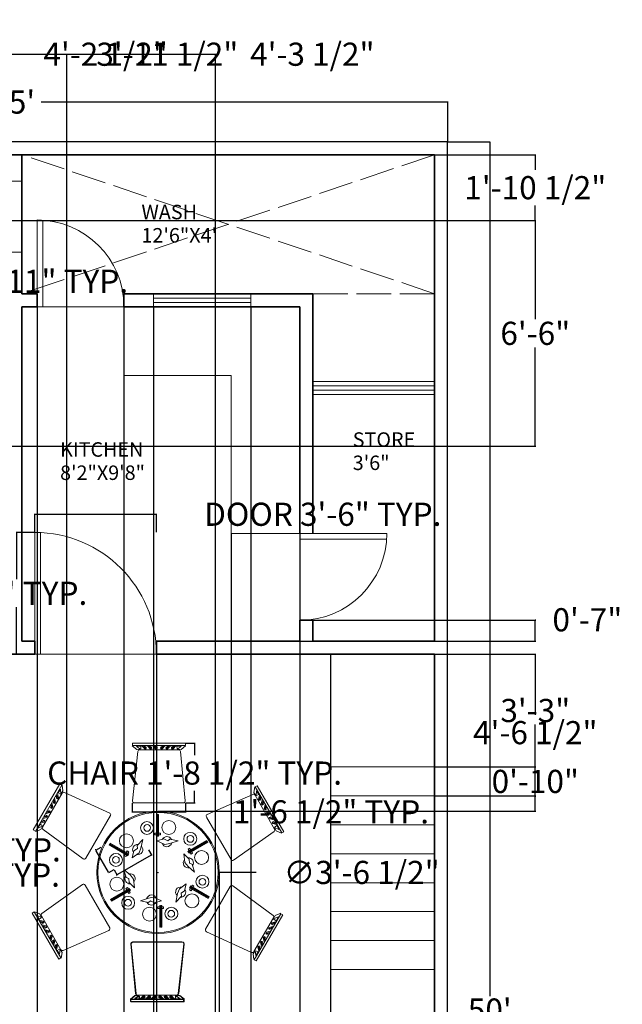
# Model space of a CAD drawing. Units: inches. Extents: x -26 to 385, y 12 to 697.
# Tile 13 of 13: x 177 to 385, y 356 to 697. Entities that reach past the tile are written whole.
import ezdxf

# ---------------------------------------------------------------- set-up
doc = ezdxf.new("R2010")
doc.units = ezdxf.units.IN
doc.header["$MEASUREMENT"] = 0
doc.linetypes.add('ACAD_ISO02W100', pattern=[15, 12, -3])
for name, color, linetype, lineweight in [('A-ANNO-DIMS', 4, 'Continuous', 18), ('A-AREA-IDEN', 4, 'Continuous', 18), ('A-DOOR', 30, 'Continuous', 20), ('A-FLOR-CASE', 7, 'Continuous', 18), ('A-FLOR-OVHD', 3, 'ACAD_ISO02W100', 13), ('A-FLOR-STRS', 215, 'Continuous', 18), ('A-GLAZ', 5, 'Continuous', 18), ('A-WALL', 40, 'Continuous', 35), ('C-PROP', 40, 'Continuous', 25), ('Furniture', 210, 'Continuous', 15)]:
    doc.layers.add(name, color=color, linetype=linetype, lineweight=lineweight)
doc.styles.get("Standard").update_dxf_attribs({"font": 'italic8.shx'})
doc.dimstyles.get("Standard").update_dxf_attribs({"dimtxt": 8, "dimasz": 0.18, "dimexe": 0.18, "dimexo": 0.0625, "dimgap": 0.09, "dimtad": 0, "dimtih": 1, "dimtoh": 1, "dimdec": 4, "dimzin": 0, "dimdsep": 46, "dimlunit": 3, "dimtxsty": 'Standard', "dimcen": 0.09, "dimclrd": 2, "dimclre": 3, "dimclrt": 6, "dimadec": 0, "dimazin": 0, "dimtfac": 1, "dimtdec": 4, "dimtofl": 0, "dimtmove": 0, "dimatfit": 3, "dimfxl": 1, "dimtolj": 1, "dimtzin": 0, "dimarcsym": 0})

# ---------------------------------------------------------------- blocks, each defined once
blk = doc.blocks.new('*D1')
at = {"layer": 'A-ANNO-DIMS', "color": 0, "lineweight": -2, "transparency": 16777216}
for p, q in [((25.13, 654.44), (25.13, 668.29)), ((25.31, 668.11), (165.52, 668.11)), ((324.95, 668.11), (184.74, 668.11)), ((325.13, 654.44), (325.13, 668.29))]:
    blk.add_line(p, q, dxfattribs=at)
at = {"layer": 'A-ANNO-DIMS', "color": 0, "transparency": 16777216}
for points in [[(25.31, 668.14), (25.31, 668.08), (25.13, 668.11)], [(324.95, 668.14), (324.95, 668.08), (325.13, 668.11)]]:
    blk.add_solid(points, dxfattribs=at)
at = {"layer": 'Defpoints', "color": 0, "transparency": 16777216}
for p in [(325.13, 668.11), (25.13, 654.38), (325.13, 654.38)]:
    blk.add_point(p, dxfattribs=at)
at = {"layer": 'A-ANNO-DIMS', "color": 0, "transparency": 16777216, "insert": (175.13, 668.11), "char_height": 8, "attachment_point": 5}
blk.add_mtext("\\A1;25'", dxfattribs=at)
blk = doc.blocks.new('*D2')
at = {"layer": 'A-ANNO-DIMS', "color": 0, "lineweight": -2, "transparency": 16777216}
for p, q in [((325.19, 654.38), (339.84, 654.38)), ((339.66, 654.2), (339.66, 359.23)), ((339.66, 54.56), (339.66, 349.53)), ((325.19, 54.38), (339.84, 54.38))]:
    blk.add_line(p, q, dxfattribs=at)
at = {"layer": 'A-ANNO-DIMS', "color": 0, "transparency": 16777216}
for points in [[(339.63, 654.2), (339.69, 654.2), (339.66, 654.38)], [(339.63, 54.56), (339.69, 54.56), (339.66, 54.38)]]:
    blk.add_solid(points, dxfattribs=at)
at = {"layer": 'Defpoints', "color": 0, "transparency": 16777216}
for p in [(325.13, 654.38), (325.13, 54.38), (339.66, 54.38)]:
    blk.add_point(p, dxfattribs=at)
at = {"layer": 'A-ANNO-DIMS', "color": 0, "transparency": 16777216, "insert": (339.66, 354.38), "char_height": 8, "attachment_point": 5}
blk.add_mtext("\\A1;50'", dxfattribs=at)
blk = doc.blocks.new('DOOR-SWING-30IN')
for p, q in [((0, -30), (0, 0)), ((0, 0), (30, 0)), ((0, -2), (30, -2))]:
    blk.add_line(p, q)
blk.add_arc((0, 0), 30, 270, 0)
blk = doc.blocks.new('DOOR-SWING-42IN')
for p, q in [((0, 0), (0, 42)), ((2, 0), (2, 42)), ((42, 0), (0, 0))]:
    blk.add_line(p, q)
blk.add_arc((0, 0), 42, 0, 90)
blk = doc.blocks.new('CHAIR-DINING')
for p, q in [((-17.53, 10.49), (-15.96, 9.24)), ((-17.41, 11.37), (-17.41, 10.56)), ((0.95, 11.37), (-17.41, 11.37)), ((-17.41, 10.56), (0.95, 10.56)), ((-16.02, 10.31), (-14.51, 10.37)), ((-14.64, 9.3), (-16.02, 10.31)), ((-14.51, 10.37), (-14.58, 9.49)), ((-14.14, 10.43), (-13.19, 9.49)), ((-13.63, 10.37), (-13.26, 10.37)), ((-12.69, 9.49), (-13.63, 10.37)), ((-13.26, 10.37), (-12.82, 9.99)), ((-12.25, 10.43), (-11.31, 9.49)), ((-11.75, 10.37), (-11.37, 10.37)), ((-10.81, 9.49), (-11.75, 10.37)), ((-11.37, 10.37), (-10.93, 9.99)), ((-10.37, 10.43), (-9.42, 9.49)), ((-9.86, 10.37), (-9.49, 10.37)), ((-8.92, 9.49), (-9.86, 10.37)), ((-9.49, 10.37), (-9.05, 9.99)), ((-7.66, 9.49), (-6.72, 10.37)), ((-7.1, 10.37), (-7.54, 9.99)), ((-6.22, 10.43), (-7.16, 9.49)), ((-6.72, 10.37), (-7.1, 10.37)), ((-5.78, 9.49), (-4.83, 10.37)), ((-5.21, 10.37), (-5.65, 9.99)), ((-4.33, 10.43), (-5.27, 9.49)), ((-4.83, 10.37), (-5.21, 10.37)), ((-3.89, 9.49), (-2.95, 10.37)), ((-3.33, 10.37), (-3.77, 9.99)), ((-2.45, 10.43), (-3.39, 9.49)), ((-2.95, 10.37), (-3.33, 10.37)), ((-2.07, 10.37), (-2.01, 9.49)), ((-0.56, 10.31), (-2.07, 10.37)), ((-1.94, 9.3), (-0.56, 10.31)), ((0.95, 10.49), (-0.62, 9.24)), ((0.95, 10.56), (0.95, 11.37)), ((-17.45, -8.54), (-15.58, 8.55)), ((-15.96, 9.24), (-14.64, 9.3)), ((-14.96, 9.11), (-1.45, 9.11)), ((-13.19, 9.49), (-12.69, 9.49)), ((-12.82, 9.99), (-12.69, 10.12)), ((-12.69, 10.12), (-12.63, 9.55)), ((-11.31, 9.49), (-10.81, 9.49)), ((-10.93, 9.99), (-10.81, 10.12)), ((-10.81, 10.12), (-10.74, 9.55)), ((-9.42, 9.49), (-8.92, 9.49)), ((-9.05, 9.99), (-8.92, 10.12)), ((-8.92, 10.12), (-8.86, 9.55)), ((-7.66, 10.12), (-7.73, 9.55)), ((-7.54, 9.99), (-7.66, 10.12)), ((-7.16, 9.49), (-7.66, 9.49)), ((-5.78, 10.12), (-5.84, 9.55)), ((-5.65, 9.99), (-5.78, 10.12)), ((-5.27, 9.49), (-5.78, 9.49)), ((-3.89, 10.12), (-3.95, 9.55)), ((-3.77, 9.99), (-3.89, 10.12)), ((-3.39, 9.49), (-3.89, 9.49)), ((-0.62, 9.24), (-1.94, 9.3)), ((-0.82, 8.54), (0.82, -8.54)), ((0.19, -9.23), (-16.83, -9.23))]:
    blk.add_line(p, q)
for centre, start, end in [((-14.96, 8.48), 90, 173.7428), ((-1.45, 8.48), 5.4801, 90), ((-16.83, -8.6), 173.7428, 270), ((0.19, -8.6), 270, 5.4801)]:
    blk.add_arc(centre, 0.629, start, end)
blk = doc.blocks.new('DINING-PLACE-SETTING')
for p, q in [((5.72, -0.56, 3.57), (-0.79, -4.32, 3.57)), ((-0.18, -3.27, 3.57), (-0.71, -3.57, 3.57)), ((-0.67, -4.53, 3.57), (5.84, -0.77, 3.57)), ((5.95, -0.95, 3.57), (-0.56, -4.71, 3.57)), ((-0.45, -4.91, 3.57), (6.06, -1.15, 3.57)), ((0.13, -3.79, 3.57), (-0.18, -3.27, 3.57)), ((5.84, -0.77, 3.57), (5.72, -0.56, 3.57)), ((6.06, -1.15, 3.57), (5.95, -0.95, 3.57)), ((-0.34, -6.97, 3.57), (-2.16, -5.22, 3.57)), ((-2.16, -5.22, 3.57), (-1.81, -8.16, 3.57)), ((-0.79, -4.32, 3.57), (-0.67, -4.53, 3.57)), ((-0.71, -3.57, 3.57), (-0.4, -4.1, 3.57)), ((-0.56, -4.71, 3.57), (-0.45, -4.91, 3.57)), ((-0.28, -4.3, 3.57), (-0.18, -4.49, 3.57)), ((-0.06, -4.69, 3.57), (0.27, -5.26, 3.57)), ((0.35, -4.18, 3.57), (0.24, -4, 3.57)), ((0.27, -5.26, 3.57), (0.8, -4.96, 3.57)), ((0.8, -4.96, 3.57), (0.47, -4.39, 3.57)), ((-1.81, -8.16, 3.57), (-0.75, -9.53, 3.57)), ((-0.75, -9.53, 3.57), (1.48, -11.52, 3.57)), ((-0.22, -8.41, 3.57), (-0.34, -6.97, 3.57)), ((0.67, -8.78, 3.57), (-0.22, -8.41, 3.57)), ((1.48, -11.52, 3.57), (0.67, -8.78, 3.57))]:
    blk.add_line(p, q)
for centre, radius in [((0, 0, 3.57), 2.24), ((0.05, -0.03, 3.57), 1.16), ((3.93, -6.44, 3.57), 2.41)]:
    blk.add_circle(centre, radius)
for start, end in [(326.6641, 94.1442), (137.0611, 284.0662)]:
    blk.add_arc((-0.65, -8.3, 3.57), 1.75, start, end)
blk = doc.blocks.new('*D13')
at = {"layer": 'A-ANNO-DIMS', "color": 3, "lineweight": -2, "transparency": 16777216}
for p, q in [((234.73, 446.56), (237.94, 446.56)), ((234.73, 425.95), (237.94, 425.95))]:
    blk.add_line(p, q, dxfattribs=at)
at = {"layer": 'A-ANNO-DIMS', "color": 2, "lineweight": -2, "transparency": 16777216}
for p, q in [((237.76, 446.38), (237.76, 442.44)), ((237.76, 426.13), (237.76, 430.07))]:
    blk.add_line(p, q, dxfattribs=at)
at = {"layer": 'A-ANNO-DIMS', "color": 2, "transparency": 16777216}
for points in [[(237.73, 446.38), (237.79, 446.38), (237.76, 446.56)], [(237.73, 426.13), (237.79, 426.13), (237.76, 425.95)]]:
    blk.add_solid(points, dxfattribs=at)
at = {"layer": 'Defpoints', "color": 0, "transparency": 16777216}
for p in [(234.67, 446.56), (237.76, 446.56), (234.67, 425.95)]:
    blk.add_point(p, dxfattribs=at)
at = {"layer": 'A-ANNO-DIMS', "color": 6, "transparency": 16777216, "insert": (237.76, 436.26), "char_height": 8, "attachment_point": 5}
blk.add_mtext('\\A1;CHAIR 1\'-8 1/2" TYP.', dxfattribs=at)
blk = doc.blocks.new('*D14')
at = {"layer": 'A-ANNO-DIMS', "color": 3, "lineweight": -2, "transparency": 16777216}
for p, q in [((216.19, 425.89), (216.19, 422.68)), ((234.67, 425.89), (234.67, 422.68))]:
    blk.add_line(p, q, dxfattribs=at)
at = {"layer": 'A-ANNO-DIMS', "color": 2, "lineweight": -2, "transparency": 16777216}
for p, q in [((216.37, 422.86), (234.49, 422.86)), ((234.67, 422.86), (234.85, 422.86))]:
    blk.add_line(p, q, dxfattribs=at)
at = {"layer": 'A-ANNO-DIMS', "color": 2, "transparency": 16777216}
for points in [[(216.37, 422.89), (216.37, 422.83), (216.19, 422.86)], [(234.49, 422.89), (234.49, 422.83), (234.67, 422.86)]]:
    blk.add_solid(points, dxfattribs=at)
at = {"layer": 'Defpoints', "color": 0, "transparency": 16777216}
for p in [(216.19, 425.95), (234.67, 425.95), (234.67, 422.86)]:
    blk.add_point(p, dxfattribs=at)
at = {"layer": 'A-ANNO-DIMS', "color": 6, "transparency": 16777216, "insert": (284.85, 422.86), "char_height": 8, "attachment_point": 5}
blk.add_mtext('\\A1;1\'-6 1/2" TYP.', dxfattribs=at)
blk = doc.blocks.new('*D15')
at = {"layer": 'A-ANNO-DIMS', "color": 3, "lineweight": -2, "transparency": 16777216}
for p, q in [((221.9, 409.73), (222.99, 407.84)), ((209.98, 402.84), (211.07, 400.96))]:
    blk.add_line(p, q, dxfattribs=at)
at = {"layer": 'A-ANNO-DIMS', "color": 2, "lineweight": -2, "transparency": 16777216}
for p, q in [((222.74, 407.9), (211.14, 401.2)), ((210.82, 401.02), (210.64, 401.02)), ((210.98, 401.11), (210.82, 401.02))]:
    blk.add_line(p, q, dxfattribs=at)
at = {"layer": 'A-ANNO-DIMS', "color": 2, "transparency": 16777216}
for points in [[(222.73, 407.93), (222.76, 407.88), (222.9, 407.99)], [(211.12, 401.23), (211.15, 401.18), (210.98, 401.11)]]:
    blk.add_solid(points, dxfattribs=at)
at = {"layer": 'Defpoints', "color": 0, "transparency": 16777216}
for p in [(221.87, 409.78), (209.95, 402.9), (210.98, 401.11)]:
    blk.add_point(p, dxfattribs=at)
at = {"layer": 'A-ANNO-DIMS', "color": 6, "transparency": 16777216, "insert": (143.32, 401.02), "char_height": 8, "attachment_point": 5}
blk.add_mtext('\\A1;SETTING 1\'-2" TYP.', dxfattribs=at)
blk = doc.blocks.new('*D16')
at = {"layer": 'A-ANNO-DIMS', "color": 2, "lineweight": -2, "transparency": 16777216}
for p, q in [((203.62, 409.73), (203.44, 409.73)), ((203.71, 409.58), (203.62, 409.73)), ((208.07, 402.02), (203.8, 409.42))]:
    blk.add_line(p, q, dxfattribs=at)
at = {"layer": 'A-ANNO-DIMS', "color": 3, "lineweight": -2, "transparency": 16777216}
for p, q in [((205.44, 410.58), (203.55, 409.49)), ((209.89, 402.87), (208, 401.78))]:
    blk.add_line(p, q, dxfattribs=at)
at = {"layer": 'A-ANNO-DIMS', "color": 2, "transparency": 16777216}
for points in [[(203.82, 409.44), (203.77, 409.41), (203.71, 409.58)], [(208.1, 402.04), (208.04, 402.01), (208.16, 401.87)]]:
    blk.add_solid(points, dxfattribs=at)
at = {"layer": 'Defpoints', "color": 0, "transparency": 16777216}
for p in [(203.71, 409.58), (205.5, 410.61), (209.95, 402.9)]:
    blk.add_point(p, dxfattribs=at)
at = {"layer": 'A-ANNO-DIMS', "color": 6, "transparency": 16777216, "insert": (167.16, 409.73), "char_height": 8, "attachment_point": 5}
blk.add_mtext('\\A1;0\'-9" TYP.', dxfattribs=at)
blk = doc.blocks.new('*D19')
at = {"layer": 'A-ANNO-DIMS', "color": 3, "lineweight": -2, "transparency": 16777216}
for p, q in [((182.59, 519.44), (182.59, 525.86)), ((224.59, 519.44), (224.59, 525.86))]:
    blk.add_line(p, q, dxfattribs=at)
at = {"layer": 'A-ANNO-DIMS', "color": 2, "lineweight": -2, "transparency": 16777216}
for p, q in [((182.77, 525.68), (224.41, 525.68)), ((224.59, 525.68), (224.77, 525.68))]:
    blk.add_line(p, q, dxfattribs=at)
at = {"layer": 'A-ANNO-DIMS', "color": 2, "transparency": 16777216}
for points in [[(182.77, 525.71), (182.77, 525.65), (182.59, 525.68)], [(224.41, 525.71), (224.41, 525.65), (224.59, 525.68)]]:
    blk.add_solid(points, dxfattribs=at)
at = {"layer": 'Defpoints', "color": 0, "transparency": 16777216}
for p in [(224.59, 525.68), (182.59, 519.38), (224.59, 519.38)]:
    blk.add_point(p, dxfattribs=at)
at = {"layer": 'A-ANNO-DIMS', "color": 6, "transparency": 16777216, "insert": (282.01, 525.68), "char_height": 8, "attachment_point": 5}
blk.add_mtext('\\A1;DOOR 3\'-6" TYP.', dxfattribs=at)
blk = doc.blocks.new('*D20')
at = {"layer": 'A-ANNO-DIMS', "color": 3, "lineweight": -2, "transparency": 16777216}
for p, q in [((182.53, 519.38), (176.11, 519.38)), ((182.53, 477.38), (176.11, 477.38))]:
    blk.add_line(p, q, dxfattribs=at)
at = {"layer": 'A-ANNO-DIMS', "color": 2, "lineweight": -2, "transparency": 16777216}
for p, q in [((176.29, 519.2), (176.29, 503.23)), ((176.29, 477.56), (176.29, 493.53))]:
    blk.add_line(p, q, dxfattribs=at)
at = {"layer": 'A-ANNO-DIMS', "color": 2, "transparency": 16777216}
for points in [[(176.26, 519.2), (176.32, 519.2), (176.29, 519.38)], [(176.26, 477.56), (176.32, 477.56), (176.29, 477.38)]]:
    blk.add_solid(points, dxfattribs=at)
at = {"layer": 'Defpoints', "color": 0, "transparency": 16777216}
for p in [(176.29, 519.38), (182.59, 519.38), (182.59, 477.38)]:
    blk.add_point(p, dxfattribs=at)
at = {"layer": 'A-ANNO-DIMS', "color": 6, "transparency": 16777216, "insert": (176.29, 498.38), "char_height": 8, "attachment_point": 5}
blk.add_mtext('\\A1;3\'-6" TYP.', dxfattribs=at)
blk = doc.blocks.new('*D21')
at = {"layer": 'A-ANNO-DIMS', "color": 3, "lineweight": -2, "transparency": 16777216}
for p, q in [((45.89, 609.6), (45.89, 606)), ((69.11, 609.6), (69.11, 606))]:
    blk.add_line(p, q, dxfattribs=at)
at = {"layer": 'A-ANNO-DIMS', "color": 2, "lineweight": -2, "transparency": 16777216}
for p, q in [((46.07, 606.18), (68.93, 606.18)), ((69.11, 606.18), (69.29, 606.18))]:
    blk.add_line(p, q, dxfattribs=at)
at = {"layer": 'A-ANNO-DIMS', "color": 2, "transparency": 16777216}
for points in [[(46.07, 606.21), (46.07, 606.15), (45.89, 606.18)], [(68.93, 606.21), (68.93, 606.15), (69.11, 606.18)]]:
    blk.add_solid(points, dxfattribs=at)
at = {"layer": 'Defpoints', "color": 0, "transparency": 16777216}
for p in [(45.89, 609.66), (69.11, 609.66), (69.11, 606.18)]:
    blk.add_point(p, dxfattribs=at)
at = {"layer": 'A-ANNO-DIMS', "color": 6, "transparency": 16777216, "insert": (152.05, 606.18), "char_height": 8, "attachment_point": 5}
blk.add_mtext('\\A1;NIGHTSTAND 1\'-11" TYP.', dxfattribs=at)
blk = doc.blocks.new('*D25')
at = {"layer": 'A-ANNO-DIMS', "color": 3, "lineweight": -2, "transparency": 16777216}
for p, q in [((284.629322, 368.316588), (284.629322, 23.949088)), ((320.629322, 368.316588), (320.629322, 23.949088))]:
    blk.add_line(p, q, dxfattribs=at)
at = {"layer": 'A-ANNO-DIMS', "color": 2, "lineweight": -2, "transparency": 16777216}
for p, q in [((284.449322, 24.129088), (284.269322, 24.129088)), ((320.809322, 24.129088), (320.989322, 24.129088))]:
    blk.add_line(p, q, dxfattribs=at)
at = {"layer": 'A-ANNO-DIMS', "color": 2, "transparency": 16777216}
for points in [[(284.449322, 24.159088), (284.449322, 24.099088), (284.629322, 24.129088)], [(320.809322, 24.159088), (320.809322, 24.099088), (320.629322, 24.129088)]]:
    blk.add_solid(points, dxfattribs=at)
at = {"layer": 'Defpoints', "color": 0, "transparency": 16777216}
for p in [(284.629322, 368.379088), (320.629322, 368.379088), (320.629322, 24.129088)]:
    blk.add_point(p, dxfattribs=at)
at = {"layer": 'A-ANNO-DIMS', "color": 6, "transparency": 16777216, "insert": (302.629322, 24.129088), "char_height": 8, "attachment_point": 5}
blk.add_mtext('\\A1;3\'-0"', dxfattribs=at)
blk = doc.blocks.new('*D26')
at = {"layer": 'A-ANNO-DIMS', "color": 3, "lineweight": -2, "transparency": 16777216}
for p, q in [((320.691822, 438.379088), (355.559322, 438.379088)), ((320.691822, 428.379088), (355.559322, 428.379088))]:
    blk.add_line(p, q, dxfattribs=at)
at = {"layer": 'A-ANNO-DIMS', "color": 2, "lineweight": -2, "transparency": 16777216}
for p, q in [((355.379322, 438.559088), (355.379322, 438.739088)), ((355.379322, 428.199088), (355.379322, 428.019088))]:
    blk.add_line(p, q, dxfattribs=at)
at = {"layer": 'A-ANNO-DIMS', "color": 2, "transparency": 16777216}
for points in [[(355.349322, 438.559088), (355.409322, 438.559088), (355.379322, 438.379088)], [(355.349322, 428.199088), (355.409322, 428.199088), (355.379322, 428.379088)]]:
    blk.add_solid(points, dxfattribs=at)
at = {"layer": 'Defpoints', "color": 0, "transparency": 16777216}
for p in [(320.629322, 438.379088), (320.629322, 428.379088), (355.379322, 428.379088)]:
    blk.add_point(p, dxfattribs=at)
at = {"layer": 'A-ANNO-DIMS', "color": 6, "transparency": 16777216, "insert": (355.379322, 433.379088), "char_height": 8, "attachment_point": 5}
blk.add_mtext('\\A1;0\'-10"', dxfattribs=at)
blk = doc.blocks.new('*D27')
at = {"layer": 'A-ANNO-DIMS', "color": 3, "lineweight": -2, "transparency": 16777216}
for p, q in [((320.69, 477.38), (355.56, 477.38)), ((320.69, 438.38), (355.56, 438.38))]:
    blk.add_line(p, q, dxfattribs=at)
at = {"layer": 'A-ANNO-DIMS', "color": 2, "lineweight": -2, "transparency": 16777216}
for p, q in [((355.38, 477.2), (355.38, 462.73)), ((355.38, 438.56), (355.38, 453.03))]:
    blk.add_line(p, q, dxfattribs=at)
at = {"layer": 'A-ANNO-DIMS', "color": 2, "transparency": 16777216}
for points in [[(355.35, 477.2), (355.41, 477.2), (355.38, 477.38)], [(355.35, 438.56), (355.41, 438.56), (355.38, 438.38)]]:
    blk.add_solid(points, dxfattribs=at)
at = {"layer": 'Defpoints', "color": 0, "transparency": 16777216}
for p in [(320.63, 477.38), (320.63, 438.38), (355.38, 438.38)]:
    blk.add_point(p, dxfattribs=at)
at = {"layer": 'A-ANNO-DIMS', "color": 6, "transparency": 16777216, "insert": (355.38, 457.88), "char_height": 8, "attachment_point": 5}
blk.add_mtext('\\A1;3\'-3"', dxfattribs=at)
blk = doc.blocks.new('*D30')
at = {"layer": 'A-ANNO-DIMS', "color": 3, "lineweight": -2, "transparency": 16777216}
for p, q in [((123.07, 627.15), (355.56, 627.15)), ((122.35, 549.23), (355.56, 549.23))]:
    blk.add_line(p, q, dxfattribs=at)
at = {"layer": 'A-ANNO-DIMS', "color": 2, "lineweight": -2, "transparency": 16777216}
for p, q in [((355.38, 626.97), (355.38, 593.04)), ((355.38, 549.41), (355.38, 583.34))]:
    blk.add_line(p, q, dxfattribs=at)
at = {"layer": 'A-ANNO-DIMS', "color": 2, "transparency": 16777216}
for points in [[(355.35, 626.97), (355.41, 626.97), (355.38, 627.15)], [(355.35, 549.41), (355.41, 549.41), (355.38, 549.23)]]:
    blk.add_solid(points, dxfattribs=at)
at = {"layer": 'Defpoints', "color": 0, "transparency": 16777216}
for p in [(123.01, 627.15), (122.29, 549.23), (355.38, 549.23)]:
    blk.add_point(p, dxfattribs=at)
at = {"layer": 'A-ANNO-DIMS', "color": 6, "transparency": 16777216, "insert": (355.38, 588.19), "char_height": 8, "attachment_point": 5}
blk.add_mtext('\\A1;6\'-6"', dxfattribs=at)
blk = doc.blocks.new('*D35')
at = {"layer": 'A-ANNO-DIMS', "color": 3, "lineweight": -2, "transparency": 16777216}
for p, q in [((193.6, 147.94), (193.6, 684.81)), ((244.99, 147.94), (244.99, 684.81))]:
    blk.add_line(p, q, dxfattribs=at)
at = {"layer": 'A-ANNO-DIMS', "color": 2, "lineweight": -2, "transparency": 16777216}
for p, q in [((193.78, 684.63), (244.81, 684.63)), ((244.99, 684.63), (245.17, 684.63))]:
    blk.add_line(p, q, dxfattribs=at)
at = {"layer": 'A-ANNO-DIMS', "color": 2, "transparency": 16777216}
for points in [[(193.78, 684.66), (193.78, 684.6), (193.6, 684.63)], [(244.81, 684.66), (244.81, 684.6), (244.99, 684.63)]]:
    blk.add_solid(points, dxfattribs=at)
at = {"layer": 'Defpoints', "color": 0, "transparency": 16777216}
for p in [(244.99, 684.63), (193.6, 147.88), (244.99, 147.88)]:
    blk.add_point(p, dxfattribs=at)
at = {"layer": 'A-ANNO-DIMS', "color": 6, "transparency": 16777216, "insert": (278.4, 684.63), "char_height": 8, "attachment_point": 5}
blk.add_mtext('\\A1;4\'-3 1/2"', dxfattribs=at)
blk = doc.blocks.new('*D36')
at = {"layer": 'A-ANNO-DIMS', "color": 3, "lineweight": -2, "transparency": 16777216}
for p, q in [((146.13, 147.94), (146.13, 684.81)), ((193.6, 147.94), (193.6, 684.81))]:
    blk.add_line(p, q, dxfattribs=at)
at = {"layer": 'A-ANNO-DIMS', "color": 2, "lineweight": -2, "transparency": 16777216}
for p, q in [((146.31, 684.63), (193.42, 684.63)), ((193.6, 684.63), (193.78, 684.63))]:
    blk.add_line(p, q, dxfattribs=at)
at = {"layer": 'A-ANNO-DIMS', "color": 2, "transparency": 16777216}
for points in [[(146.31, 684.66), (146.31, 684.6), (146.13, 684.63)], [(193.42, 684.66), (193.42, 684.6), (193.6, 684.63)]]:
    blk.add_solid(points, dxfattribs=at)
at = {"layer": 'Defpoints', "color": 0, "transparency": 16777216}
for p in [(193.6, 684.63), (146.13, 147.88), (193.6, 147.88)]:
    blk.add_point(p, dxfattribs=at)
at = {"layer": 'A-ANNO-DIMS', "color": 6, "transparency": 16777216, "insert": (228.34, 684.63), "char_height": 8, "attachment_point": 5}
blk.add_mtext('\\A1;3\'-11 1/2"', dxfattribs=at)
blk = doc.blocks.new('*D37')
at = {"layer": 'A-ANNO-DIMS', "color": 3, "lineweight": -2, "transparency": 16777216}
for p, q in [((223.55, 597.32), (223.55, 23.95)), ((257.22, 597.32), (257.22, 23.95))]:
    blk.add_line(p, q, dxfattribs=at)
at = {"layer": 'A-ANNO-DIMS', "color": 2, "lineweight": -2, "transparency": 16777216}
for p, q in [((223.73, 24.13), (257.04, 24.13)), ((257.22, 24.13), (257.4, 24.13))]:
    blk.add_line(p, q, dxfattribs=at)
at = {"layer": 'A-ANNO-DIMS', "color": 2, "transparency": 16777216}
for points in [[(223.73, 24.16), (223.73, 24.1), (223.55, 24.13)], [(257.04, 24.16), (257.04, 24.1), (257.22, 24.13)]]:
    blk.add_solid(points, dxfattribs=at)
at = {"layer": 'Defpoints', "color": 0, "transparency": 16777216}
for p in [(223.55, 597.38), (257.22, 597.38), (257.22, 24.13)]:
    blk.add_point(p, dxfattribs=at)
at = {"layer": 'A-ANNO-DIMS', "color": 6, "transparency": 16777216, "insert": (290.63, 24.13), "char_height": 8, "attachment_point": 5}
blk.add_mtext('\\A1;2\'-9 1/2"', dxfattribs=at)
blk = doc.blocks.new('*D39')
at = {"layer": 'A-ANNO-DIMS', "color": 3, "lineweight": -2, "transparency": 16777216}
for p, q in [((183.36, 597.32), (183.36, 23.95)), ((213.36, 597.32), (213.36, 23.95))]:
    blk.add_line(p, q, dxfattribs=at)
at = {"layer": 'A-ANNO-DIMS', "color": 2, "lineweight": -2, "transparency": 16777216}
for p, q in [((183.54, 24.13), (213.18, 24.13)), ((213.36, 24.13), (213.54, 24.13))]:
    blk.add_line(p, q, dxfattribs=at)
at = {"layer": 'A-ANNO-DIMS', "color": 2, "transparency": 16777216}
for points in [[(183.54, 24.16), (183.54, 24.1), (183.36, 24.13)], [(213.18, 24.16), (213.18, 24.1), (213.36, 24.13)]]:
    blk.add_solid(points, dxfattribs=at)
at = {"layer": 'Defpoints', "color": 0, "transparency": 16777216}
for p in [(183.36, 597.38), (213.36, 597.38), (213.36, 24.13)]:
    blk.add_point(p, dxfattribs=at)
at = {"layer": 'A-ANNO-DIMS', "color": 6, "transparency": 16777216, "insert": (231.53, 24.13), "char_height": 8, "attachment_point": 5}
blk.add_mtext('\\A1;2\'-6"', dxfattribs=at)
blk = doc.blocks.new('*D42')
at = {"layer": 'A-ANNO-DIMS', "color": 3, "lineweight": -2, "transparency": 16777216}
for p, q in [((250.37, 518.99), (250.37, 23.95)), ((274.13, 518.99), (274.13, 23.95))]:
    blk.add_line(p, q, dxfattribs=at)
at = {"layer": 'A-ANNO-DIMS', "color": 2, "lineweight": -2, "transparency": 16777216}
for p, q in [((250.55, 24.13), (273.95, 24.13)), ((274.13, 24.13), (274.31, 24.13))]:
    blk.add_line(p, q, dxfattribs=at)
at = {"layer": 'A-ANNO-DIMS', "color": 2, "transparency": 16777216}
for points in [[(250.55, 24.16), (250.55, 24.1), (250.37, 24.13)], [(273.95, 24.16), (273.95, 24.1), (274.13, 24.13)]]:
    blk.add_solid(points, dxfattribs=at)
at = {"layer": 'Defpoints', "color": 0, "transparency": 16777216}
for p in [(250.37, 519.05), (274.13, 519.05), (274.13, 24.13)]:
    blk.add_point(p, dxfattribs=at)
at = {"layer": 'A-ANNO-DIMS', "color": 6, "transparency": 16777216, "insert": (292.3, 24.13), "char_height": 8, "attachment_point": 5}
blk.add_mtext('\\A1;2\'-0"', dxfattribs=at)
blk = doc.blocks.new('*D44')
at = {"layer": 'A-ANNO-DIMS', "color": 3, "lineweight": -2, "transparency": 16777216}
for p, q in [((274.19, 489.05), (355.56, 489.05)), ((274.19, 481.88), (355.56, 481.88))]:
    blk.add_line(p, q, dxfattribs=at)
at = {"layer": 'A-ANNO-DIMS', "color": 2, "lineweight": -2, "transparency": 16777216}
for p, q in [((355.38, 489.05), (355.38, 489.23)), ((355.38, 489.23), (355.56, 489.23)), ((355.38, 482.06), (355.38, 488.87))]:
    blk.add_line(p, q, dxfattribs=at)
at = {"layer": 'A-ANNO-DIMS', "color": 2, "transparency": 16777216}
for points in [[(355.35, 488.87), (355.41, 488.87), (355.38, 489.05)], [(355.35, 482.06), (355.41, 482.06), (355.38, 481.88)]]:
    blk.add_solid(points, dxfattribs=at)
at = {"layer": 'Defpoints', "color": 0, "transparency": 16777216}
for p in [(274.13, 489.05), (355.38, 489.05), (274.13, 481.88)]:
    blk.add_point(p, dxfattribs=at)
at = {"layer": 'A-ANNO-DIMS', "color": 6, "transparency": 16777216, "insert": (373.36, 489.23), "char_height": 8, "attachment_point": 5}
blk.add_mtext('\\A1;0\'-7"', dxfattribs=at)
blk = doc.blocks.new('*D46')
at = {"layer": 'A-ANNO-DIMS', "color": 3, "lineweight": -2, "transparency": 16777216}
for p, q in [((224.59, 477.32), (224.59, 23.95)), ((284.63, 477.32), (284.63, 23.95))]:
    blk.add_line(p, q, dxfattribs=at)
at = {"layer": 'A-ANNO-DIMS', "color": 2, "lineweight": -2, "transparency": 16777216}
for p, q in [((224.77, 24.13), (236.62, 24.13)), ((284.45, 24.13), (272.61, 24.13))]:
    blk.add_line(p, q, dxfattribs=at)
at = {"layer": 'A-ANNO-DIMS', "color": 2, "transparency": 16777216}
for points in [[(224.77, 24.16), (224.77, 24.1), (224.59, 24.13)], [(284.45, 24.16), (284.45, 24.1), (284.63, 24.13)]]:
    blk.add_solid(points, dxfattribs=at)
at = {"layer": 'Defpoints', "color": 0, "transparency": 16777216}
for p in [(224.59, 477.38), (284.63, 477.38), (284.63, 24.13)]:
    blk.add_point(p, dxfattribs=at)
at = {"layer": 'A-ANNO-DIMS', "color": 6, "transparency": 16777216, "insert": (254.61, 24.13), "char_height": 8, "attachment_point": 5}
blk.add_mtext('\\A1;5\'-0"', dxfattribs=at)
blk = doc.blocks.new('*D48')
at = {"layer": 'A-ANNO-DIMS', "color": 3, "lineweight": -2, "transparency": 16777216}
for p, q in [((123.01, 627.21), (123.01, 684.81)), ((173.63, 649.94), (173.63, 684.81))]:
    blk.add_line(p, q, dxfattribs=at)
at = {"layer": 'A-ANNO-DIMS', "color": 2, "lineweight": -2, "transparency": 16777216}
for p, q in [((123.19, 684.63), (173.45, 684.63)), ((173.63, 684.63), (173.81, 684.63))]:
    blk.add_line(p, q, dxfattribs=at)
at = {"layer": 'A-ANNO-DIMS', "color": 2, "transparency": 16777216}
for points in [[(123.19, 684.66), (123.19, 684.6), (123.01, 684.63)], [(173.45, 684.66), (173.45, 684.6), (173.63, 684.63)]]:
    blk.add_solid(points, dxfattribs=at)
at = {"layer": 'Defpoints', "color": 0, "transparency": 16777216}
for p in [(173.63, 684.63), (173.63, 649.88), (123.01, 627.15)]:
    blk.add_point(p, dxfattribs=at)
at = {"layer": 'A-ANNO-DIMS', "color": 6, "transparency": 16777216, "insert": (207.04, 684.63), "char_height": 8, "attachment_point": 5}
blk.add_mtext('\\A1;4\'-2 1/2"', dxfattribs=at)
blk = doc.blocks.new('*D49')
at = {"layer": 'A-ANNO-DIMS', "color": 3, "lineweight": -2, "transparency": 16777216}
for p, q in [((173.69, 649.88), (355.56, 649.88)), ((123.07, 627.15), (355.56, 627.15))]:
    blk.add_line(p, q, dxfattribs=at)
at = {"layer": 'A-ANNO-DIMS', "color": 2, "lineweight": -2, "transparency": 16777216}
for p, q in [((355.38, 649.7), (355.38, 644.7)), ((355.38, 627.33), (355.38, 632.33))]:
    blk.add_line(p, q, dxfattribs=at)
at = {"layer": 'A-ANNO-DIMS', "color": 2, "transparency": 16777216}
for points in [[(355.35, 649.7), (355.41, 649.7), (355.38, 649.88)], [(355.35, 627.33), (355.41, 627.33), (355.38, 627.15)]]:
    blk.add_solid(points, dxfattribs=at)
at = {"layer": 'Defpoints', "color": 0, "transparency": 16777216}
for p in [(173.63, 649.88), (355.38, 649.88), (123.01, 627.15)]:
    blk.add_point(p, dxfattribs=at)
at = {"layer": 'A-ANNO-DIMS', "color": 6, "transparency": 16777216, "insert": (355.38, 638.52), "char_height": 8, "attachment_point": 5}
blk.add_mtext('\\A1;1\'-10 1/2"', dxfattribs=at)
blk = doc.blocks.new('*D50')
at = {"layer": 'A-ANNO-DIMS', "color": 3, "lineweight": -2, "transparency": 16777216}
for p, q in [((246.28, 401.87), (246.28, 23.95)), ((284.63, 398.32), (284.63, 23.95))]:
    blk.add_line(p, q, dxfattribs=at)
at = {"layer": 'A-ANNO-DIMS', "color": 2, "lineweight": -2, "transparency": 16777216}
for p, q in [((246.46, 24.13), (284.45, 24.13)), ((284.63, 24.13), (284.81, 24.13))]:
    blk.add_line(p, q, dxfattribs=at)
at = {"layer": 'A-ANNO-DIMS', "color": 2, "transparency": 16777216}
for points in [[(246.46, 24.16), (246.46, 24.1), (246.28, 24.13)], [(284.45, 24.16), (284.45, 24.1), (284.63, 24.13)]]:
    blk.add_solid(points, dxfattribs=at)
at = {"layer": 'Defpoints', "color": 0, "transparency": 16777216}
for p in [(246.28, 401.93), (284.63, 398.38), (284.63, 24.13)]:
    blk.add_point(p, dxfattribs=at)
at = {"layer": 'A-ANNO-DIMS', "color": 6, "transparency": 16777216, "insert": (318.04, 24.13), "char_height": 8, "attachment_point": 5}
blk.add_mtext('\\A1;3\'-2 1/2"', dxfattribs=at)
blk = doc.blocks.new('*D51')
at = {"layer": 'A-ANNO-DIMS', "color": 3, "lineweight": -2, "transparency": 16777216}
for p, q in [((224.66, 477.38), (355.56, 477.38)), ((225.2, 423.08), (355.56, 423.08))]:
    blk.add_line(p, q, dxfattribs=at)
at = {"layer": 'A-ANNO-DIMS', "color": 2, "lineweight": -2, "transparency": 16777216}
for p, q in [((355.38, 477.2), (355.38, 456.41)), ((355.38, 423.26), (355.38, 444.04))]:
    blk.add_line(p, q, dxfattribs=at)
at = {"layer": 'A-ANNO-DIMS', "color": 2, "transparency": 16777216}
for points in [[(355.35, 477.2), (355.41, 477.2), (355.38, 477.38)], [(355.35, 423.26), (355.41, 423.26), (355.38, 423.08)]]:
    blk.add_solid(points, dxfattribs=at)
at = {"layer": 'Defpoints', "color": 0, "transparency": 16777216}
for p in [(224.59, 477.38), (355.38, 477.38), (225.14, 423.08)]:
    blk.add_point(p, dxfattribs=at)
at = {"layer": 'A-ANNO-DIMS', "color": 6, "transparency": 16777216, "insert": (355.38, 450.23), "char_height": 8, "attachment_point": 5}
blk.add_mtext('\\A1;4\'-6 1/2"', dxfattribs=at)
blk = doc.blocks.new('*D56')
at = {"layer": 'A-ANNO-DIMS', "color": 3, "lineweight": -2, "transparency": 16777216}
for p, q in [((225.05, 401.93), (225.23, 401.93)), ((225.14, 401.84), (225.14, 402.02))]:
    blk.add_line(p, q, dxfattribs=at)
at = {"layer": 'A-ANNO-DIMS', "color": 2, "lineweight": -2, "transparency": 16777216}
blk.add_line((258.96, 401.93), (246.46, 401.93), dxfattribs=at)
at = {"layer": 'A-ANNO-DIMS', "color": 2, "transparency": 16777216}
blk.add_solid([(246.46, 401.96), (246.46, 401.9), (246.28, 401.93)], dxfattribs=at)
at = {"layer": 'Defpoints', "color": 0, "transparency": 16777216}
for p in [(203.99, 401.93), (246.28, 401.93)]:
    blk.add_point(p, dxfattribs=at)
at = {"layer": 'A-ANNO-DIMS', "color": 6, "transparency": 16777216, "insert": (295.43, 401.93), "char_height": 8, "attachment_point": 5}
blk.add_mtext('\\A1;∅3\'-6 1/2"', dxfattribs=at)

msp = doc.modelspace()

# ---------------------------------------------------------------- linework, layer by layer
at = {"layer": 'A-DOOR'}
for p, q in [((183.35855, 597.37909), (183.35855, 627.37909)), ((185.35855, 597.37909), (185.35855, 627.24582)), ((213.35855, 597.37909), (183.35855, 597.37909))]:
    msp.add_line(p, q, dxfattribs=at)
msp.add_arc((183.35855, 597.37909), 30, 360, 90, dxfattribs=at)
at = {"layer": 'A-FLOR-CASE'}
for p, q in [((213.35855, 597.37909), (213.35855, 573.64862)), ((213.35855, 573.64862), (250.37102, 573.64862)), ((250.37102, 573.64862), (250.37102, 519.05498)), ((250.37102, 519.05498), (278.62932, 519.05498))]:
    msp.add_line(p, q, dxfattribs=at)
at = {"layer": 'A-FLOR-OVHD'}
for p, q in [((320.62932, 601.87909), (178.12932, 649.87909)), ((320.62932, 649.87909), (178.12932, 601.87909)), ((278.62932, 601.87909), (320.62932, 601.87909))]:
    msp.add_line(p, q, dxfattribs=at)
at = {"layer": 'A-FLOR-STRS'}
for p, q in [((284.62932, 327.87909), (284.62932, 477.37909)), ((320.62932, 438.37909), (284.62932, 438.37909)), ((320.62932, 428.37909), (284.62932, 428.37909)), ((320.62932, 418.37909), (284.62932, 418.37909)), ((320.62932, 408.37909), (284.62932, 408.37909)), ((320.62932, 398.37909), (284.62932, 398.37909)), ((320.62932, 388.37909), (284.62932, 388.37909)), ((320.62932, 378.37909), (284.62932, 378.37909)), ((320.62932, 368.37909), (284.62932, 368.37909))]:
    msp.add_line(p, q, dxfattribs=at)
at = {"layer": 'A-GLAZ'}
for p, q in [((178.12932, 640.78173), (173.62932, 640.78173)), ((178.12932, 616.22584), (178.12932, 640.78173)), ((173.62932, 616.22584), (178.12932, 616.22584)), ((223.54856, 601.87909), (223.54856, 597.37909)), ((257.21981, 601.87909), (223.54856, 601.87909)), ((223.54856, 600.37909), (257.21981, 600.37909)), ((223.54856, 598.87909), (257.21981, 598.87909)), ((257.21981, 597.37909), (257.21981, 601.87909)), ((223.54856, 597.37909), (257.21981, 597.37909)), ((278.62932, 571.52804), (320.62932, 571.52804)), ((278.62932, 567.02804), (278.62932, 571.52804)), ((320.62932, 571.52804), (320.62932, 567.02804)), ((278.62932, 570.02804), (320.62932, 570.02804)), ((278.62932, 568.52804), (320.62932, 568.52804)), ((320.62932, 567.02804), (278.62932, 567.02804))]:
    msp.add_line(p, q, dxfattribs=at)
at = {"layer": 'A-WALL'}
for p, q in [((320.62932, 649.87909), (29.62932, 649.87909)), ((178.12932, 649.87909), (178.12932, 601.87909)), ((320.62932, 481.87909), (320.62932, 649.87909)), ((183.35855, 601.87909), (178.12932, 601.87909)), ((183.35855, 601.87909), (183.35855, 597.37909)), ((278.62932, 601.87909), (213.35855, 601.87909)), ((213.35855, 601.87909), (213.35855, 597.37909)), ((278.62932, 519.05498), (278.62932, 601.87909)), ((178.12932, 597.37909), (178.12932, 481.87909)), ((183.35855, 597.37909), (178.12932, 597.37909)), ((274.12932, 597.37909), (213.35855, 597.37909)), ((274.12932, 519.05498), (274.12932, 597.37909)), ((274.12932, 481.87909), (274.12932, 489.05498)), ((278.62932, 489.05498), (274.12932, 489.05498)), ((278.62932, 481.87909), (278.62932, 489.05498)), ((182.59493, 481.87909), (178.12932, 481.87909)), ((182.59493, 481.87909), (182.59493, 477.37909)), ((274.12932, 481.87909), (224.59493, 481.87909)), ((224.59493, 481.87909), (224.59493, 477.37909)), ((320.62932, 481.87909), (278.62932, 481.87909)), ((182.59493, 477.37909), (168.19858, 477.37909)), ((320.62932, 477.37909), (224.59493, 477.37909)), ((320.62932, 332.37909), (320.62932, 477.37909))]:
    msp.add_line(p, q, dxfattribs=at)
at = {"layer": 'C-PROP'}
for p, q in [((325.12932, 654.37909), (25.12932, 654.37909)), ((325.12932, 54.37909), (325.12932, 654.37909))]:
    msp.add_line(p, q, dxfattribs=at)
at = {"layer": 'Furniture'}
for radius in [21.14266, 20.74896]:
    msp.add_circle((225.13562, 401.934), radius, dxfattribs=at)

# ---------------------------------------------------------------- block references
at = {"layer": 'A-DOOR'}
for name, p in [('DOOR-SWING-42IN', (182.59493, 477.37909)), ('DOOR-SWING-30IN', (274.12932, 519.05498))]:
    msp.add_blockref(name, p, dxfattribs=at)
at = {"layer": 'Furniture'}
for name, p in [('CHAIR-DINING', (233.7225, 435.1865)), ('DINING-PLACE-SETTING', (236.24914, 413.5355))]:
    msp.add_blockref(name, p, dxfattribs=at)
for name, p, rotation in [('CHAIR-DINING', (200.63155, 425.99671), 59.99999999999278), ('CHAIR-DINING', (258.22657, 411.12379), 300.0000000000035), ('DINING-PLACE-SETTING', (221.32259, 417.28765), 59.99999999999342), ('DINING-PLACE-SETTING', (210.60986, 406.23695), 120.0000000000015), ('DINING-PLACE-SETTING', (214.82368, 391.4341), 180), ('DINING-PLACE-SETTING', (240.46296, 398.73266), 299.9999999999992), ('CHAIR-DINING', (192.04467, 392.7442), 120.0000000000036), ('DINING-PLACE-SETTING', (229.75023, 387.68196), 239.9999999999942), ('CHAIR-DINING', (249.63969, 377.87129), 240.0000000000072), ('CHAIR-DINING', (216.54874, 368.68149), 180), ('CHAIR-DINING', (216.71083, 368.62175), 180)]:
    msp.add_blockref(name, p, dxfattribs=dict(at, rotation=rotation))

# ---------------------------------------------------------------- texts
at = {"layer": 'A-AREA-IDEN'}
for s, p in [('WASH', (219.41899, 627.60025)), ('12\'6"X4\'', (219.41899, 619.56819)), ('STORE', (292.36175, 548.98992)), ('KITCHEN', (191.32132, 545.56667)), ('3\'6"', (292.36175, 540.95786)), ('8\'2"X9\'8"', (191.32132, 537.53461))]:
    msp.add_text(s, height=5, dxfattribs=at).set_placement(p)

# ---------------------------------------------------------------- dimensions: what is measured, and where the dimension line sits
at = {"layer": 'A-ANNO-DIMS'}
for base, p1, p2, override, picture, middle in [((173.62932, 684.62909), (123.00609, 627.15179), (173.62932, 649.87909), {"dimdec": 1, "dimlfac": 1, "dimrnd": 0, "dimzin": 1, "dimdsep": 46, "dimlunit": 4, "dimfrac": 2}, '*D48', (207.04218, 684.62909)), ((193.59818, 684.62909), (146.12932, 147.87909), (193.59818, 147.87909), {"dimdec": 1, "dimlfac": 1, "dimrnd": 0, "dimzin": 1, "dimdsep": 46, "dimlunit": 4, "dimfrac": 2}, '*D36', (228.34437, 684.62909)), ((244.98557, 684.62909), (193.59818, 147.87909), (244.98557, 147.87909), {"dimdec": 1, "dimlfac": 1, "dimrnd": 0, "dimzin": 1, "dimdsep": 46, "dimlunit": 4, "dimfrac": 2}, '*D35', (278.39843, 684.62909)), ((325.12932, 668.10538), (25.12932, 654.37909), (325.12932, 654.37909), {"dimclrd": 0, "dimclre": 0, "dimclrt": 0}, '*D1', (175.12932, 668.10538)), ((213.35855, 24.12909), (183.35855, 597.37909), (213.35855, 597.37909), {"dimdec": 1, "dimlfac": 1, "dimrnd": 0, "dimzin": 1, "dimdsep": 46, "dimlunit": 4, "dimfrac": 2}, '*D39', (231.53331, 24.12909)), ((257.21981, 24.12909), (223.54856, 597.37909), (257.21981, 597.37909), {"dimdec": 1, "dimlfac": 1, "dimrnd": 0, "dimzin": 1, "dimdsep": 46, "dimlunit": 4, "dimfrac": 2}, '*D37', (290.63267, 24.12909)), ((274.12932, 24.12909), (250.37102, 519.05498), (274.12932, 519.05498), {"dimdec": 1, "dimlfac": 1, "dimrnd": 0, "dimzin": 1, "dimdsep": 46, "dimlunit": 4, "dimfrac": 2}, '*D42', (292.30408, 24.12909)), ((284.62932, 24.12909), (224.59493, 477.37909), (284.62932, 477.37909), {"dimdec": 1, "dimlfac": 1, "dimrnd": 0, "dimzin": 1, "dimdsep": 46, "dimlunit": 4, "dimfrac": 2}, '*D46', (254.61213, 24.12909)), ((284.62932, 24.12909), (246.27828, 401.934), (284.62932, 398.37909), {"dimdec": 1, "dimlfac": 1, "dimrnd": 0, "dimzin": 1, "dimdsep": 46, "dimlunit": 4, "dimfrac": 2}, '*D50', (318.04218, 24.12909)), ((320.62932, 24.12909), (284.62932, 368.37909), (320.62932, 368.37909), {"dimdec": 1, "dimlfac": 1, "dimrnd": 0, "dimzin": 1, "dimdsep": 46, "dimlunit": 4, "dimfrac": 2}, '*D25', (302.62932, 24.12909))]:
    dim = msp.add_linear_dim(base=base, p1=p1, p2=p2, dimstyle='Standard', override=override, dxfattribs=at)
    dim.commit()
    dim.dimension.update_dxf_attribs({"geometry": picture, "text_midpoint": middle})
for base, p1, p2, override, picture, middle in [((339.65968, 54.37909), (325.12932, 654.37909), (325.12932, 54.37909), {"dimclrd": 0, "dimclre": 0, "dimclrt": 0}, '*D2', (339.65968, 354.37909)), ((355.37932, 649.87909), (123.00609, 627.15179), (173.62932, 649.87909), {"dimdec": 1, "dimlfac": 1, "dimrnd": 0, "dimzin": 1, "dimdsep": 46, "dimlunit": 4, "dimfrac": 2}, '*D49', (355.37932, 638.51544)), ((355.37932, 549.23099), (123.00609, 627.15179), (122.28508, 549.23099), {"dimdec": 1, "dimlfac": 1, "dimrnd": 0, "dimzin": 1, "dimdsep": 46, "dimlunit": 4, "dimfrac": 2}, '*D30', (355.37932, 588.19139)), ((355.37932, 489.05498), (274.12932, 481.87909), (274.12932, 489.05498), {"dimdec": 1, "dimlfac": 1, "dimrnd": 0, "dimzin": 1, "dimdsep": 46, "dimlunit": 4, "dimfrac": 2}, '*D44', (373.36361, 489.23498)), ((355.37932, 477.37909), (225.13562, 423.07666), (224.59493, 477.37909), {"dimdec": 1, "dimlfac": 1, "dimrnd": 0, "dimzin": 1, "dimdsep": 46, "dimlunit": 4, "dimfrac": 2}, '*D51', (355.37932, 450.22787)), ((355.37932, 438.37909), (320.62932, 477.37909), (320.62932, 438.37909), {"dimdec": 1, "dimlfac": 1, "dimrnd": 0, "dimzin": 1, "dimdsep": 46, "dimlunit": 4, "dimfrac": 2}, '*D27', (355.37932, 457.87909)), ((355.37932, 428.37909), (320.62932, 438.37909), (320.62932, 428.37909), {"dimdec": 1, "dimlfac": 1, "dimrnd": 0, "dimzin": 1, "dimdsep": 46, "dimlunit": 4, "dimfrac": 2}, '*D26', (355.37932, 433.37909))]:
    dim = msp.add_linear_dim(base=base, p1=p1, p2=p2, angle=90, dimstyle='Standard', override=override, dxfattribs=at)
    dim.commit()
    dim.dimension.update_dxf_attribs({"geometry": picture, "text_midpoint": middle})
for base, p1, p2, text, picture, middle in [((69.11284, 606.17509), (45.88754, 609.65889), (69.11284, 609.65889), 'NIGHTSTAND <> TYP.', '*D21', (152.04951, 606.17509)), ((224.59493, 525.67909), (182.59493, 519.37909), (224.59493, 519.37909), 'DOOR <> TYP.', '*D19', (282.00779, 525.67909)), ((234.67083, 422.86343), (216.19179, 425.95427), (234.67083, 425.95427), '<> TYP.', '*D14', (284.84559, 422.86343))]:
    dim = msp.add_linear_dim(base=base, p1=p1, p2=p2, text=text, dimstyle='Standard', override={"dimdec": 1, "dimlfac": 1, "dimrnd": 0, "dimzin": 1, "dimdsep": 46, "dimlunit": 4, "dimfrac": 2}, dxfattribs=at)
    dim.commit()
    dim.dimension.update_dxf_attribs({"geometry": picture, "text_midpoint": middle})
for base, p1, p2, angle, text, picture, middle in [((176.29493, 519.37909), (182.59493, 477.37909), (182.59493, 519.37909), 90, '<> TYP.', '*D20', (176.29493, 498.37909)), ((237.76168, 446.55993), (234.67083, 425.95427), (234.67083, 446.55993), 90, 'CHAIR <> TYP.', '*D13', (237.76168, 436.2571)), ((210.98037, 401.11114), (221.86605, 409.77955), (209.94826, 402.8988), 210, 'SETTING <> TYP.', '*D15', (143.31639, 401.02114)), ((203.70876, 409.57749), (209.94826, 402.8988), (205.49643, 410.6096), 120, '<> TYP.', '*D16', (167.15828, 409.73337))]:
    dim = msp.add_linear_dim(base=base, p1=p1, p2=p2, angle=angle, text=text, dimstyle='Standard', override={"dimdec": 1, "dimlfac": 1, "dimrnd": 0, "dimzin": 1, "dimdsep": 46, "dimlunit": 4, "dimfrac": 2}, dxfattribs=at)
    dim.commit()
    dim.dimension.update_dxf_attribs({"geometry": picture, "text_midpoint": middle})
dim = msp.add_diameter_dim_2p(p1=(203.99296, 401.93399), p2=(246.27828, 401.934), dimstyle='Standard', override={"dimdec": 1, "dimlfac": 1, "dimrnd": 0, "dimzin": 1, "dimdsep": 46, "dimlunit": 4, "dimfrac": 2}, dxfattribs=at)
dim.commit()
dim.dimension.update_dxf_attribs({"geometry": '*D56', "text_midpoint": (258.96388, 401.934), "dimtype": 163})

doc.saveas('drawing.dxf')
